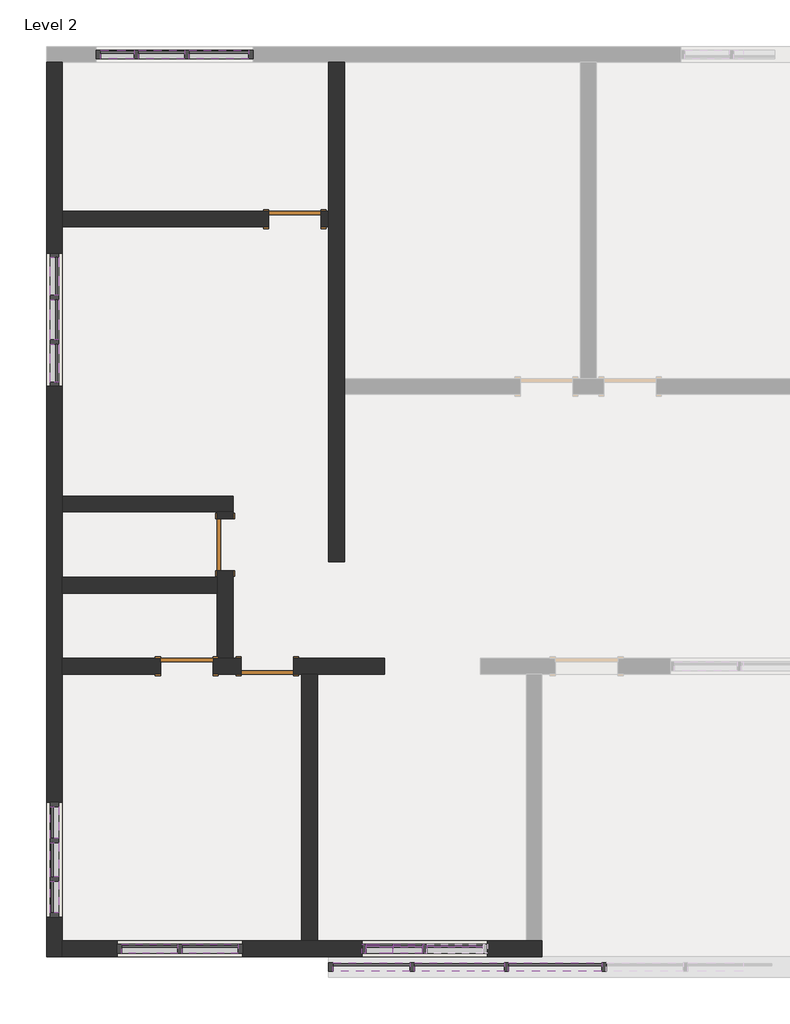
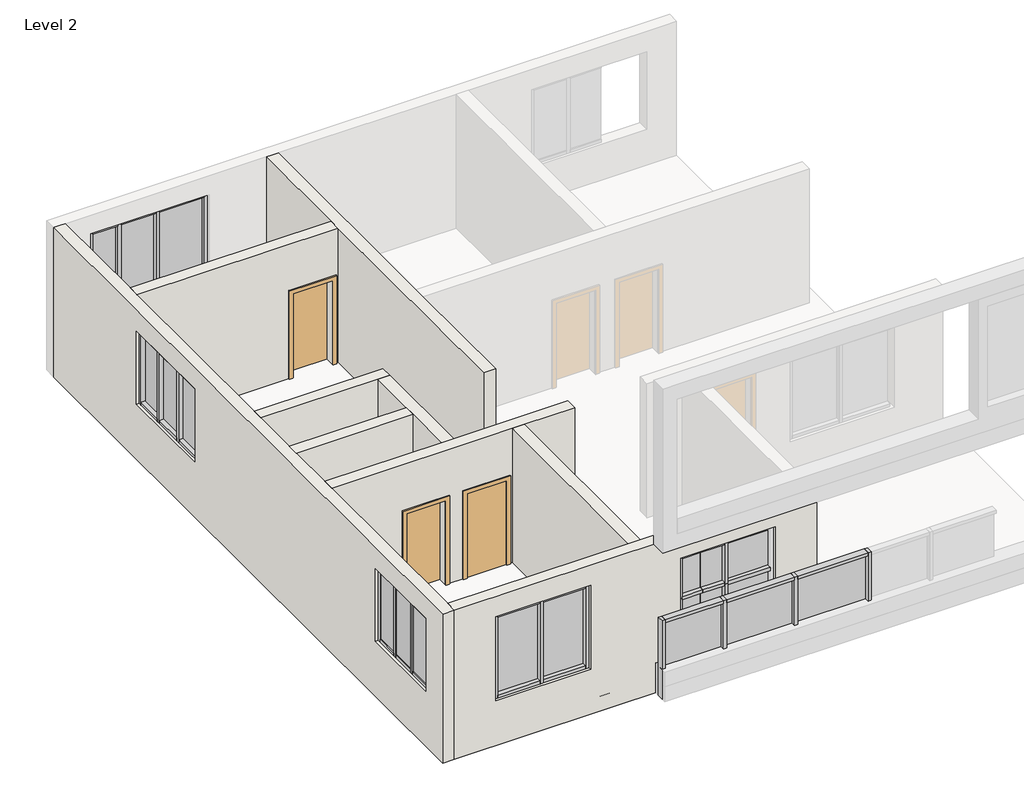
# One storey, part 1 of 2: 56 members, 20 plates, 9 walls, 4 doors.
"""IFC4 building model written with IfcOpenShell, lengths in millimetres."""

from ifc_helpers import new_model, si_unit, frame, origin, place, context, project, spatial, polyline, outline, extrude, faceted_brep, transform, mapped, element, save
from components import door_a1484949, door_85036156, member_c17f1be2, member_ad567e07, member_5535eeb3, member_2ebf4a73, member_b9f3750b, member_051277f3, member_024c663a, member_e254c550, member_3fd136ac, member_73c075c8, member_623bfa76, member_6049e8cb, member_177cc448, member_bc64557a, member_c85333fa, member_70b87a21, member_5e57c25a, member_84b97a81, member_951753a7, member_7096a90e, member_0adfe7f4, member_3d200c31, member_5d841d64, member_75b26f99, member_e6b9f524, member_001188f2, member_d37749d9, member_0d0414c4, system_panel_glazed_b96e00cd, system_panel_glazed_b203cd48, system_panel_glazed_f5076819, system_panel_glazed_6dadbfa4, system_panel_glazed_18fdb1ad, system_panel_glazed_5b9b0e9e, system_panel_glazed_bdb83165, system_panel_glazed_79b80f84, system_panel_glazed_c1c9c451, system_panel_glazed_831e08d1, system_panel_glazed_30877d7e, system_panel_glazed_de05bfa4, system_panel_glazed_4af92da9, system_panel_glazed_616dcef8

model = new_model("IFC4")

# Units and contexts
model_context = context("Model", 3, world=origin())
ifc_project = project(units=[si_unit("LENGTHUNIT", "METRE", prefix="MILLI")], contexts=[model_context])

# Site, building, storey
site = spatial("IfcSite", under=ifc_project)
building = spatial("IfcBuilding", under=site)
storey = spatial("IfcBuildingStorey", under=building, Name="Level 2", Elevation=3048.0)

# Doors
placement = place(None, origin())
door_shape = door_a1484949(model_context)
element("IfcDoor", 1, ObjectType="Single-Flush : 30\" x 80\"", at=placement, inside=storey, context=model_context, shape_type="MappedRepresentation", body=[
    mapped(door_shape, transform((-16666.091855, -3109.9538163, 3048.0), x_axis=(1.0, 0.0, 0.0), y_axis=(0.0, 1.0, 0.0), z_axis=(0.0, 0.0, 1.0))),
])
element("IfcDoor", 2, ObjectType="Single-Flush : 30\" x 80\"", at=placement, inside=storey, context=model_context, shape_type="MappedRepresentation", body=[
    mapped(door_shape, transform((-18240.891855, -9625.0538163, 3048.0), x_axis=(1.0, 0.0, 0.0), y_axis=(0.0, 1.0, 0.0), z_axis=(0.0, 0.0, 1.0))),
])
door_2_shape = door_85036156(model_context)
element("IfcDoor", 3, ObjectType="Single-Flush : 30\" x 80\"", at=placement, inside=storey, context=model_context, shape_type="MappedRepresentation", body=[
    mapped(door_2_shape, transform((-17682.091855, -7853.4038163, 3048.0), x_axis=(0.0, -1.0, 0.0), y_axis=(1.0, 0.0, 0.0), z_axis=(0.0, 0.0, 1.0))),
])
element("IfcDoor", 4, ObjectType="Single-Flush : 30\" x 80\"", at=placement, inside=storey, context=model_context, shape_type="MappedRepresentation", body=[
    mapped(door_2_shape, transform((-17066.141855, -9625.0538163, 3048.0), x_axis=(1.0, 0.0, 0.0), y_axis=(0.0, 1.0, 0.0), z_axis=(0.0, 0.0, 1.0))),
])

# Members
member_shape = member_c17f1be2(model_context)
element("IfcMember", 5, ObjectType="Rectangular Mullion : 2.5\" x 5\" rectangular", at=placement, inside=storey, context=model_context, shape_type="MappedRepresentation", body=[
    mapped(member_shape, transform((-18374.241855, -13739.8538163, 5684.1406455), x_axis=(0.0, 0.0, 1.0), y_axis=(0.0, -1.0, 0.0), z_axis=(1.0, 0.0, 0.0))),
])
element("IfcMember", 6, ObjectType="Rectangular Mullion : 2.5\" x 5\" rectangular", at=placement, inside=storey, context=model_context, shape_type="MappedRepresentation", body=[
    mapped(member_shape, transform((-17491.591855, -13739.8538163, 5684.1406455), x_axis=(0.0, 0.0, 1.0), y_axis=(0.0, -1.0, 0.0), z_axis=(1.0, 0.0, 0.0))),
])
member_2_shape = member_ad567e07(model_context)
element("IfcMember", 7, ObjectType="Rectangular Mullion : 2.5\" x 5\" rectangular", at=placement, inside=storey, context=model_context, shape_type="MappedRepresentation", body=[
    mapped(member_2_shape, transform((-13922.891855, -13739.8538163, 4760.0253323), x_axis=(0.0, 0.0, 1.0), y_axis=(0.0, -1.0, 0.0), z_axis=(1.0, 0.0, 0.0))),
])
element("IfcMember", 8, ObjectType="Rectangular Mullion : 2.5\" x 5\" rectangular", at=placement, inside=storey, context=model_context, shape_type="MappedRepresentation", body=[
    mapped(member_shape, transform((-14742.041855, -13739.8538163, 3888.7401376), x_axis=(0.0, 0.0, -1.0), y_axis=(0.0, -1.0, 0.0), z_axis=(-1.0, 0.0, 0.0))),
])
element("IfcMember", 9, ObjectType="Rectangular Mullion : 2.5\" x 5\" rectangular", at=placement, inside=storey, context=model_context, shape_type="MappedRepresentation", body=[
    mapped(member_shape, transform((-18310.741855, -13739.8538163, 3967.0387154), x_axis=(0.0, 0.0, -1.0), y_axis=(0.0, -1.0, 0.0), z_axis=(-1.0, 0.0, 0.0))),
])
element("IfcMember", 10, ObjectType="Rectangular Mullion : 2.5\" x 5\" rectangular", at=placement, inside=storey, context=model_context, shape_type="MappedRepresentation", body=[
    mapped(member_shape, transform((-19193.391855, -13739.8538163, 3967.0387154), x_axis=(0.0, 0.0, -1.0), y_axis=(0.0, -1.0, 0.0), z_axis=(-1.0, 0.0, 0.0))),
])
member_3_shape = member_5535eeb3(model_context)
element("IfcMember", 11, ObjectType="Rectangular Mullion : 2.5\" x 5\" rectangular", at=placement, inside=storey, context=model_context, shape_type="MappedRepresentation", body=[
    mapped(member_3_shape, transform((-20171.291855, -12755.6038163, 5664.075508), x_axis=(0.0, 0.0, 1.0), y_axis=(1.0, 0.0, 0.0), z_axis=(0.0, 1.0, 0.0))),
])
element("IfcMember", 12, ObjectType="Rectangular Mullion : 2.5\" x 5\" rectangular", at=placement, inside=storey, context=model_context, shape_type="MappedRepresentation", body=[
    mapped(member_3_shape, transform((-20171.291855, -11669.7538163, 5664.075508), x_axis=(0.0, 0.0, 1.0), y_axis=(1.0, 0.0, 0.0), z_axis=(0.0, 1.0, 0.0))),
])
member_4_shape = member_2ebf4a73(model_context)
element("IfcMember", 13, ObjectType="Rectangular Mullion : 2.5\" x 5\" rectangular", at=placement, inside=storey, context=model_context, shape_type="MappedRepresentation", body=[
    mapped(member_4_shape, transform((-20171.291855, -12196.8038163, 5664.075508), x_axis=(0.0, 0.0, 1.0), y_axis=(1.0, 0.0, 0.0), z_axis=(0.0, 1.0, 0.0))),
])
element("IfcMember", 14, ObjectType="Rectangular Mullion : 2.5\" x 5\" rectangular", at=placement, inside=storey, context=model_context, shape_type="MappedRepresentation", body=[
    mapped(member_4_shape, transform((-20171.291855, -12692.1038163, 4177.2250348), x_axis=(0.0, 0.0, -1.0), y_axis=(1.0, 0.0, 0.0), z_axis=(0.0, -1.0, 0.0))),
])
element("IfcMember", 15, ObjectType="Rectangular Mullion : 2.5\" x 5\" rectangular", at=placement, inside=storey, context=model_context, shape_type="MappedRepresentation", body=[
    mapped(member_3_shape, transform((-20171.291855, -12133.3038163, 4177.2250348), x_axis=(0.0, 0.0, -1.0), y_axis=(1.0, 0.0, 0.0), z_axis=(0.0, -1.0, 0.0))),
])
element("IfcMember", 16, ObjectType="Rectangular Mullion : 2.5\" x 5\" rectangular", at=placement, inside=storey, context=model_context, shape_type="MappedRepresentation", body=[
    mapped(member_3_shape, transform((-20171.291855, -13219.1538163, 4177.2250348), x_axis=(0.0, 0.0, -1.0), y_axis=(1.0, 0.0, 0.0), z_axis=(0.0, -1.0, 0.0))),
])
member_5_shape = member_b9f3750b(model_context)
element("IfcMember", 17, ObjectType="Rectangular Mullion : 2.5\" x 5\" rectangular", at=placement, inside=storey, context=model_context, shape_type="MappedRepresentation", body=[
    mapped(member_5_shape, transform((-19009.241855, -709.6538163, 5710.0962507), x_axis=(0.0, 0.0, 1.0), y_axis=(0.0, -1.0, 0.0), z_axis=(1.0, 0.0, 0.0))),
])
member_6_shape = member_051277f3(model_context)
element("IfcMember", 18, ObjectType="Rectangular Mullion : 2.5\" x 5\" rectangular", at=placement, inside=storey, context=model_context, shape_type="MappedRepresentation", body=[
    mapped(member_6_shape, transform((-18272.641855, -709.6538163, 5710.0962507), x_axis=(0.0, 0.0, 1.0), y_axis=(0.0, -1.0, 0.0), z_axis=(1.0, 0.0, 0.0))),
])
member_7_shape = member_024c663a(model_context)
element("IfcMember", 19, ObjectType="Rectangular Mullion : 2.5\" x 5\" rectangular", at=placement, inside=storey, context=model_context, shape_type="MappedRepresentation", body=[
    mapped(member_7_shape, transform((-17339.191855, -709.6538163, 5710.0962507), x_axis=(0.0, 0.0, 1.0), y_axis=(0.0, -1.0, 0.0), z_axis=(1.0, 0.0, 0.0))),
])
member_8_shape = member_e254c550(model_context)
element("IfcMember", 20, ObjectType="Rectangular Mullion : 2.5\" x 5\" rectangular", at=placement, inside=storey, context=model_context, shape_type="MappedRepresentation", body=[
    mapped(member_8_shape, transform((-18240.891855, -709.6538163, 4156.5855814), x_axis=(1.0, 0.0, 0.0), y_axis=(0.0, -1.0, 0.0), z_axis=(0.0, 0.0, -1.0))),
])
element("IfcMember", 21, ObjectType="Rectangular Mullion : 2.5\" x 5\" rectangular", at=placement, inside=storey, context=model_context, shape_type="MappedRepresentation", body=[
    mapped(member_8_shape, transform((-18977.491855, -709.6538163, 4156.5855814), x_axis=(1.0, 0.0, 0.0), y_axis=(0.0, -1.0, 0.0), z_axis=(0.0, 0.0, -1.0))),
])
element("IfcMember", 22, ObjectType="Rectangular Mullion : 2.5\" x 5\" rectangular", at=placement, inside=storey, context=model_context, shape_type="MappedRepresentation", body=[
    mapped(member_6_shape, transform((-18945.741855, -709.6538163, 4156.5855814), x_axis=(0.0, 0.0, -1.0), y_axis=(0.0, -1.0, 0.0), z_axis=(-1.0, 0.0, 0.0))),
])
element("IfcMember", 23, ObjectType="Rectangular Mullion : 2.5\" x 5\" rectangular", at=placement, inside=storey, context=model_context, shape_type="MappedRepresentation", body=[
    mapped(member_7_shape, transform((-18209.141855, -709.6538163, 4156.5855814), x_axis=(0.0, 0.0, -1.0), y_axis=(0.0, -1.0, 0.0), z_axis=(-1.0, 0.0, 0.0))),
])
element("IfcMember", 24, ObjectType="Rectangular Mullion : 2.5\" x 5\" rectangular", at=placement, inside=storey, context=model_context, shape_type="MappedRepresentation", body=[
    mapped(member_5_shape, transform((-19498.191855, -709.6538163, 4156.5855814), x_axis=(0.0, 0.0, -1.0), y_axis=(0.0, -1.0, 0.0), z_axis=(-1.0, 0.0, 0.0))),
])
member_9_shape = member_3fd136ac(model_context)
element("IfcMember", 25, ObjectType="Rectangular Mullion : 2.5\" x 5\" rectangular", at=placement, inside=storey, context=model_context, shape_type="MappedRepresentation", body=[
    mapped(member_9_shape, transform((-19561.691855, -709.6538163, 5710.0962507), x_axis=(-1.0, 0.0, 0.0), y_axis=(0.0, -1.0, 0.0), z_axis=(0.0, 0.0, 1.0))),
])
element("IfcMember", 26, ObjectType="Rectangular Mullion : 2.5\" x 5\" rectangular", at=placement, inside=storey, context=model_context, shape_type="MappedRepresentation", body=[
    mapped(member_9_shape, transform((-17275.691855, -709.6538163, 4156.5855814), x_axis=(1.0, 0.0, 0.0), y_axis=(0.0, -1.0, 0.0), z_axis=(0.0, 0.0, -1.0))),
])
member_10_shape = member_73c075c8(model_context)
element("IfcMember", 27, ObjectType="Rectangular Mullion : 2.5\" x 5\" rectangular", at=placement, inside=storey, context=model_context, shape_type="MappedRepresentation", body=[
    mapped(member_10_shape, transform((-20171.291855, -4932.4038163, 4168.0644408), x_axis=(0.0, 0.0, -1.0), y_axis=(-1.0, 0.0, 0.0), z_axis=(0.0, 1.0, 0.0))),
])
element("IfcMember", 28, ObjectType="Rectangular Mullion : 2.5\" x 5\" rectangular", at=placement, inside=storey, context=model_context, shape_type="MappedRepresentation", body=[
    mapped(member_10_shape, transform((-20171.291855, -3668.7538163, 4168.0644408), x_axis=(0.0, 0.0, -1.0), y_axis=(-1.0, 0.0, 0.0), z_axis=(0.0, 1.0, 0.0))),
])
member_11_shape = member_623bfa76(model_context)
element("IfcMember", 29, ObjectType="Rectangular Mullion : 2.5\" x 5\" rectangular", at=placement, inside=storey, context=model_context, shape_type="MappedRepresentation", body=[
    mapped(member_11_shape, transform((-20171.291855, -4284.7038163, 4168.0644408), x_axis=(0.0, 0.0, -1.0), y_axis=(-1.0, 0.0, 0.0), z_axis=(0.0, 1.0, 0.0))),
])
member_12_shape = member_6049e8cb(model_context)
element("IfcMember", 30, ObjectType="Rectangular Mullion : 2.5\" x 5\" rectangular", at=placement, inside=storey, context=model_context, shape_type="MappedRepresentation", body=[
    mapped(member_12_shape, transform((-20171.291855, -4900.6538163, 4168.0644408), x_axis=(0.0, -1.0, 0.0), y_axis=(-1.0, 0.0, 0.0), z_axis=(0.0, 0.0, -1.0))),
])
element("IfcMember", 31, ObjectType="Rectangular Mullion : 2.5\" x 5\" rectangular", at=placement, inside=storey, context=model_context, shape_type="MappedRepresentation", body=[
    mapped(member_12_shape, transform((-20171.291855, -4252.9538163, 4168.0644408), x_axis=(0.0, -1.0, 0.0), y_axis=(-1.0, 0.0, 0.0), z_axis=(0.0, 0.0, -1.0))),
])
element("IfcMember", 32, ObjectType="Rectangular Mullion : 2.5\" x 5\" rectangular", at=placement, inside=storey, context=model_context, shape_type="MappedRepresentation", body=[
    mapped(member_11_shape, transform((-20171.291855, -4868.9038163, 5661.6118891), x_axis=(0.0, 0.0, 1.0), y_axis=(-1.0, 0.0, 0.0), z_axis=(0.0, -1.0, 0.0))),
])
element("IfcMember", 33, ObjectType="Rectangular Mullion : 2.5\" x 5\" rectangular", at=placement, inside=storey, context=model_context, shape_type="MappedRepresentation", body=[
    mapped(member_10_shape, transform((-20171.291855, -4221.2038163, 5661.6118891), x_axis=(0.0, 0.0, 1.0), y_axis=(-1.0, 0.0, 0.0), z_axis=(0.0, -1.0, 0.0))),
])
element("IfcMember", 34, ObjectType="Rectangular Mullion : 2.5\" x 5\" rectangular", at=placement, inside=storey, context=model_context, shape_type="MappedRepresentation", body=[
    mapped(member_10_shape, transform((-20171.291855, -5484.8538163, 5661.6118891), x_axis=(0.0, 0.0, 1.0), y_axis=(-1.0, 0.0, 0.0), z_axis=(0.0, -1.0, 0.0))),
])
member_13_shape = member_177cc448(model_context)
element("IfcMember", 35, ObjectType="Rectangular Mullion : 2.5\" x 5\" rectangular", at=placement, inside=storey, context=model_context, shape_type="MappedRepresentation", body=[
    mapped(member_13_shape, transform((-20171.291855, -5548.3538163, 4168.0644408), x_axis=(0.0, -1.0, 0.0), y_axis=(-1.0, 0.0, 0.0), z_axis=(0.0, 0.0, -1.0))),
])
element("IfcMember", 36, ObjectType="Rectangular Mullion : 2.5\" x 5\" rectangular", at=placement, inside=storey, context=model_context, shape_type="MappedRepresentation", body=[
    mapped(member_13_shape, transform((-20171.291855, -3605.2538163, 5661.6118891), x_axis=(0.0, 1.0, 0.0), y_axis=(-1.0, 0.0, 0.0), z_axis=(0.0, 0.0, 1.0))),
])
member_14_shape = member_bc64557a(model_context)
element("IfcMember", 37, ObjectType="Rectangular Mullion : 2.5\" x 5\" rectangular", at=placement, inside=storey, context=model_context, shape_type="MappedRepresentation", body=[
    mapped(member_14_shape, transform((-20171.291855, -12165.0538163, 4177.2250348), x_axis=(0.0, 1.0, 0.0), y_axis=(1.0, 0.0, 0.0), z_axis=(0.0, 0.0, -1.0))),
])
element("IfcMember", 38, ObjectType="Rectangular Mullion : 2.5\" x 5\" rectangular", at=placement, inside=storey, context=model_context, shape_type="MappedRepresentation", body=[
    mapped(member_14_shape, transform((-20171.291855, -12723.8538163, 4177.2250348), x_axis=(0.0, 1.0, 0.0), y_axis=(1.0, 0.0, 0.0), z_axis=(0.0, 0.0, -1.0))),
])
member_15_shape = member_c85333fa(model_context)
element("IfcMember", 39, ObjectType="Rectangular Mullion : 2.5\" x 5\" rectangular", at=placement, inside=storey, context=model_context, shape_type="MappedRepresentation", body=[
    mapped(member_15_shape, transform((-20171.291855, -13282.6538163, 5664.075508), x_axis=(0.0, -1.0, 0.0), y_axis=(1.0, 0.0, 0.0), z_axis=(0.0, 0.0, 1.0))),
])
element("IfcMember", 40, ObjectType="Rectangular Mullion : 2.5\" x 5\" rectangular", at=placement, inside=storey, context=model_context, shape_type="MappedRepresentation", body=[
    mapped(member_15_shape, transform((-20171.291855, -11606.2538163, 4177.2250348), x_axis=(0.0, 1.0, 0.0), y_axis=(1.0, 0.0, 0.0), z_axis=(0.0, 0.0, -1.0))),
])
member_16_shape = member_70b87a21(model_context)
element("IfcMember", 41, ObjectType="Rectangular Mullion : 2.5\" x 5\" rectangular", at=placement, inside=storey, context=model_context, shape_type="MappedRepresentation", body=[
    mapped(member_16_shape, transform((-14805.541855, -13739.8538163, 4760.0253323), x_axis=(0.0, 0.0, 1.0), y_axis=(0.0, -1.0, 0.0), z_axis=(1.0, 0.0, 0.0))),
])
member_17_shape = member_5e57c25a(model_context)
element("IfcMember", 42, ObjectType="Rectangular Mullion : 2.5\" x 5\" rectangular", at=placement, inside=storey, context=model_context, shape_type="MappedRepresentation", body=[
    mapped(member_17_shape, transform((-14773.791855, -13739.8538163, 4760.0253323), x_axis=(1.0, 0.0, 0.0), y_axis=(0.0, -1.0, 0.0), z_axis=(0.0, 0.0, -1.0))),
])
member_18_shape = member_84b97a81(model_context)
element("IfcMember", 43, ObjectType="Rectangular Mullion : 2.5\" x 5\" rectangular", at=placement, inside=storey, context=model_context, shape_type="MappedRepresentation", body=[
    mapped(member_18_shape, transform((-14805.541855, -13739.8538163, 5631.310527), x_axis=(0.0, 0.0, 1.0), y_axis=(0.0, -1.0, 0.0), z_axis=(1.0, 0.0, 0.0))),
])
element("IfcMember", 44, ObjectType="Rectangular Mullion : 2.5\" x 5\" rectangular", at=placement, inside=storey, context=model_context, shape_type="MappedRepresentation", body=[
    mapped(member_17_shape, transform((-14773.791855, -13739.8538163, 3888.7401376), x_axis=(1.0, 0.0, 0.0), y_axis=(0.0, -1.0, 0.0), z_axis=(0.0, 0.0, -1.0))),
])
element("IfcMember", 45, ObjectType="Rectangular Mullion : 2.5\" x 5\" rectangular", at=placement, inside=storey, context=model_context, shape_type="MappedRepresentation", body=[
    mapped(member_18_shape, transform((-15230.991855, -13739.8538163, 3888.7401376), x_axis=(0.0, 0.0, -1.0), y_axis=(0.0, -1.0, 0.0), z_axis=(-1.0, 0.0, 0.0))),
])
member_19_shape = member_951753a7(model_context)
element("IfcMember", 46, ObjectType="Rectangular Mullion : 2.5\" x 5\" rectangular", at=placement, inside=storey, context=model_context, shape_type="MappedRepresentation", body=[
    mapped(member_19_shape, transform((-15230.991855, -13739.8538163, 4760.0253323), x_axis=(0.0, 0.0, 1.0), y_axis=(0.0, -1.0, 0.0), z_axis=(1.0, 0.0, 0.0))),
])
member_20_shape = member_7096a90e(model_context)
element("IfcMember", 47, ObjectType="Rectangular Mullion : 2.5\" x 5\" rectangular", at=placement, inside=storey, context=model_context, shape_type="MappedRepresentation", body=[
    mapped(member_20_shape, transform((-15230.991855, -13739.8538163, 5631.310527), x_axis=(0.0, 0.0, 1.0), y_axis=(0.0, -1.0, 0.0), z_axis=(1.0, 0.0, 0.0))),
])
element("IfcMember", 48, ObjectType="Rectangular Mullion : 2.5\" x 5\" rectangular", at=placement, inside=storey, context=model_context, shape_type="MappedRepresentation", body=[
    mapped(member_20_shape, transform((-15624.691855, -13739.8538163, 3888.7401376), x_axis=(0.0, 0.0, -1.0), y_axis=(0.0, -1.0, 0.0), z_axis=(-1.0, 0.0, 0.0))),
])
member_21_shape = member_0adfe7f4(model_context)
element("IfcMember", 49, ObjectType="Rectangular Mullion : 2.5\" x 5\" rectangular", at=placement, inside=storey, context=model_context, shape_type="MappedRepresentation", body=[
    mapped(member_21_shape, transform((-15688.191855, -13739.8538163, 4760.0253323), x_axis=(-1.0, 0.0, 0.0), y_axis=(0.0, -1.0, 0.0), z_axis=(0.0, 0.0, 1.0))),
])
element("IfcMember", 50, ObjectType="Rectangular Mullion : 2.5\" x 5\" rectangular", at=placement, inside=storey, context=model_context, shape_type="MappedRepresentation", body=[
    mapped(member_21_shape, transform((-15688.191855, -13739.8538163, 5631.310527), x_axis=(-1.0, 0.0, 0.0), y_axis=(0.0, -1.0, 0.0), z_axis=(0.0, 0.0, 1.0))),
])
member_22_shape = member_3d200c31(model_context)
element("IfcMember", 51, ObjectType="Rectangular Mullion : 2.5\" x 5\" rectangular", at=placement, inside=storey, context=model_context, shape_type="MappedRepresentation", body=[
    mapped(member_22_shape, transform((-18342.491855, -13739.8538163, 3967.0387154), x_axis=(1.0, 0.0, 0.0), y_axis=(0.0, -1.0, 0.0), z_axis=(0.0, 0.0, -1.0))),
])
member_23_shape = member_5d841d64(model_context)
element("IfcMember", 52, ObjectType="Rectangular Mullion : 2.5\" x 5\" rectangular", at=placement, inside=storey, context=model_context, shape_type="MappedRepresentation", body=[
    mapped(member_23_shape, transform((-17428.091855, -13739.8538163, 3967.0387154), x_axis=(1.0, 0.0, 0.0), y_axis=(0.0, -1.0, 0.0), z_axis=(0.0, 0.0, -1.0))),
])
element("IfcMember", 53, ObjectType="Rectangular Mullion : 2.5\" x 5\" rectangular", at=placement, inside=storey, context=model_context, shape_type="MappedRepresentation", body=[
    mapped(member_23_shape, transform((-19256.891855, -13739.8538163, 5684.1406455), x_axis=(-1.0, 0.0, 0.0), y_axis=(0.0, -1.0, 0.0), z_axis=(0.0, 0.0, 1.0))),
])
member_24_shape = member_75b26f99(model_context)
element("IfcMember", 54, ObjectType="Rectangular Mullion : 2.5\" x 5\" rectangular", at=placement, inside=storey, context=model_context, shape_type="MappedRepresentation", body=[
    mapped(member_24_shape, transform((-16170.791855, -14006.5538163, 4647.2829369), x_axis=(-1.0, 0.0, 0.0), y_axis=(0.0, -1.0, 0.0), z_axis=(0.0, 0.0, 1.0))),
])
member_25_shape = member_e6b9f524(model_context)
element("IfcMember", 55, ObjectType="Rectangular Mullion : 2.5\" x 5\" rectangular", at=placement, inside=storey, context=model_context, shape_type="MappedRepresentation", body=[
    mapped(member_25_shape, transform((-14983.341855, -14006.5538163, 4647.2829369), x_axis=(0.0, 0.0, 1.0), y_axis=(0.0, -1.0, 0.0), z_axis=(1.0, 0.0, 0.0))),
])
member_26_shape = member_001188f2(model_context)
element("IfcMember", 56, ObjectType="Rectangular Mullion : 2.5\" x 5\" rectangular", at=placement, inside=storey, context=model_context, shape_type="MappedRepresentation", body=[
    mapped(member_26_shape, transform((-14951.591855, -14006.5538163, 3048.0), x_axis=(1.0, 0.0, 0.0), y_axis=(0.0, -1.0, 0.0), z_axis=(0.0, 0.0, -1.0))),
])
element("IfcMember", 57, ObjectType="Rectangular Mullion : 2.5\" x 5\" rectangular", at=placement, inside=storey, context=model_context, shape_type="MappedRepresentation", body=[
    mapped(member_26_shape, transform((-13579.991855, -14006.5538163, 3048.0), x_axis=(1.0, 0.0, 0.0), y_axis=(0.0, -1.0, 0.0), z_axis=(0.0, 0.0, -1.0))),
])
element("IfcMember", 58, ObjectType="Rectangular Mullion : 2.5\" x 5\" rectangular", at=placement, inside=storey, context=model_context, shape_type="MappedRepresentation", body=[
    mapped(member_26_shape, transform((-12157.591855, -14006.5538163, 3048.0), x_axis=(1.0, 0.0, 0.0), y_axis=(0.0, -1.0, 0.0), z_axis=(0.0, 0.0, -1.0))),
])
member_27_shape = member_d37749d9(model_context)
element("IfcMember", 59, ObjectType="Rectangular Mullion : 2.5\" x 5\" rectangular", at=placement, inside=storey, context=model_context, shape_type="MappedRepresentation", body=[
    mapped(member_27_shape, transform((-13611.741855, -14006.5538163, 4647.2829369), x_axis=(0.0, 0.0, 1.0), y_axis=(0.0, -1.0, 0.0), z_axis=(1.0, 0.0, 0.0))),
])
member_28_shape = member_0d0414c4(model_context)
element("IfcMember", 60, ObjectType="Rectangular Mullion : 2.5\" x 5\" rectangular", at=placement, inside=storey, context=model_context, shape_type="MappedRepresentation", body=[
    mapped(member_28_shape, transform((-12189.341855, -14006.5538163, 4647.2829369), x_axis=(0.0, 0.0, 1.0), y_axis=(0.0, -1.0, 0.0), z_axis=(1.0, 0.0, 0.0))),
])

# Plates
system_panel_glazed_shape = system_panel_glazed_b96e00cd(model_context)
element("IfcPlate", 61, ObjectType="System Panel : Glazed", at=placement, inside=storey, context=model_context, shape_type="MappedRepresentation", body=[
    mapped(system_panel_glazed_shape, transform((-19253.716855, -709.6538163, 4220.0855814), x_axis=(1.0, 0.0, 0.0), y_axis=(0.0, 1.0, 0.0), z_axis=(0.0, 0.0, 1.0))),
])
system_panel_glazed_2_shape = system_panel_glazed_b203cd48(model_context)
element("IfcPlate", 62, ObjectType="System Panel : Glazed", at=placement, inside=storey, context=model_context, shape_type="MappedRepresentation", body=[
    mapped(system_panel_glazed_2_shape, transform((-17774.166855, -709.6538163, 4220.0855814), x_axis=(1.0, 0.0, 0.0), y_axis=(0.0, 1.0, 0.0), z_axis=(0.0, 0.0, 1.0))),
])
system_panel_glazed_3_shape = system_panel_glazed_f5076819(model_context)
element("IfcPlate", 63, ObjectType="System Panel : Glazed", at=placement, inside=storey, context=model_context, shape_type="MappedRepresentation", body=[
    mapped(system_panel_glazed_3_shape, transform((-18609.191855, -709.6538163, 4220.0855814), x_axis=(1.0, 0.0, 0.0), y_axis=(0.0, 1.0, 0.0), z_axis=(0.0, 0.0, 1.0))),
])
system_panel_glazed_4_shape = system_panel_glazed_6dadbfa4(model_context)
element("IfcPlate", 64, ObjectType="System Panel : Glazed", at=placement, inside=storey, context=model_context, shape_type="MappedRepresentation", body=[
    mapped(system_panel_glazed_4_shape, transform((-20171.291855, -3944.9788163, 4231.5644408), x_axis=(0.0, -1.0, 0.0), y_axis=(1.0, 0.0, 0.0), z_axis=(0.0, 0.0, 1.0))),
])
element("IfcPlate", 65, ObjectType="System Panel : Glazed", at=placement, inside=storey, context=model_context, shape_type="MappedRepresentation", body=[
    mapped(system_panel_glazed_4_shape, transform((-20171.291855, -5208.6288163, 4231.5644408), x_axis=(0.0, -1.0, 0.0), y_axis=(1.0, 0.0, 0.0), z_axis=(0.0, 0.0, 1.0))),
])
system_panel_glazed_5_shape = system_panel_glazed_18fdb1ad(model_context)
element("IfcPlate", 66, ObjectType="System Panel : Glazed", at=placement, inside=storey, context=model_context, shape_type="MappedRepresentation", body=[
    mapped(system_panel_glazed_5_shape, transform((-20171.291855, -4576.8038163, 4231.5644408), x_axis=(0.0, -1.0, 0.0), y_axis=(1.0, 0.0, 0.0), z_axis=(0.0, 0.0, 1.0))),
])
system_panel_glazed_6_shape = system_panel_glazed_5b9b0e9e(model_context)
element("IfcPlate", 67, ObjectType="System Panel : Glazed", at=placement, inside=storey, context=model_context, shape_type="MappedRepresentation", body=[
    mapped(system_panel_glazed_6_shape, transform((-20171.291855, -12987.3788163, 4240.7250348), x_axis=(0.0, 1.0, 0.0), y_axis=(-1.0, 0.0, 0.0), z_axis=(0.0, 0.0, 1.0))),
])
element("IfcPlate", 68, ObjectType="System Panel : Glazed", at=placement, inside=storey, context=model_context, shape_type="MappedRepresentation", body=[
    mapped(system_panel_glazed_6_shape, transform((-20171.291855, -11901.5288163, 4240.7250348), x_axis=(0.0, 1.0, 0.0), y_axis=(-1.0, 0.0, 0.0), z_axis=(0.0, 0.0, 1.0))),
])
system_panel_glazed_7_shape = system_panel_glazed_bdb83165(model_context)
element("IfcPlate", 69, ObjectType="System Panel : Glazed", at=placement, inside=storey, context=model_context, shape_type="MappedRepresentation", body=[
    mapped(system_panel_glazed_7_shape, transform((-20171.291855, -12444.4538163, 4240.7250348), x_axis=(0.0, 1.0, 0.0), y_axis=(-1.0, 0.0, 0.0), z_axis=(0.0, 0.0, 1.0))),
])
system_panel_glazed_8_shape = system_panel_glazed_79b80f84(model_context)
element("IfcPlate", 70, ObjectType="System Panel : Glazed", at=placement, inside=storey, context=model_context, shape_type="MappedRepresentation", body=[
    mapped(system_panel_glazed_8_shape, transform((-15018.266855, -13739.8538163, 3952.2401376), x_axis=(1.0, 0.0, 0.0), y_axis=(0.0, 1.0, 0.0), z_axis=(0.0, 0.0, 1.0))),
])
element("IfcPlate", 71, ObjectType="System Panel : Glazed", at=placement, inside=storey, context=model_context, shape_type="MappedRepresentation", body=[
    mapped(system_panel_glazed_8_shape, transform((-15018.266855, -13739.8538163, 4791.7753323), x_axis=(1.0, 0.0, 0.0), y_axis=(0.0, 1.0, 0.0), z_axis=(0.0, 0.0, 1.0))),
])
system_panel_glazed_9_shape = system_panel_glazed_c1c9c451(model_context)
element("IfcPlate", 72, ObjectType="System Panel : Glazed", at=placement, inside=storey, context=model_context, shape_type="MappedRepresentation", body=[
    mapped(system_panel_glazed_9_shape, transform((-14332.466855, -13739.8538163, 3952.2401376), x_axis=(1.0, 0.0, 0.0), y_axis=(0.0, 1.0, 0.0), z_axis=(0.0, 0.0, 1.0))),
])
element("IfcPlate", 73, ObjectType="System Panel : Glazed", at=placement, inside=storey, context=model_context, shape_type="MappedRepresentation", body=[
    mapped(system_panel_glazed_9_shape, transform((-14332.466855, -13739.8538163, 4791.7753323), x_axis=(1.0, 0.0, 0.0), y_axis=(0.0, 1.0, 0.0), z_axis=(0.0, 0.0, 1.0))),
])
system_panel_glazed_10_shape = system_panel_glazed_831e08d1(model_context)
element("IfcPlate", 74, ObjectType="System Panel : Glazed", at=placement, inside=storey, context=model_context, shape_type="MappedRepresentation", body=[
    mapped(system_panel_glazed_10_shape, transform((-15427.841855, -13739.8538163, 3952.2401376), x_axis=(1.0, 0.0, 0.0), y_axis=(0.0, 1.0, 0.0), z_axis=(0.0, 0.0, 1.0))),
])
element("IfcPlate", 75, ObjectType="System Panel : Glazed", at=placement, inside=storey, context=model_context, shape_type="MappedRepresentation", body=[
    mapped(system_panel_glazed_10_shape, transform((-15427.841855, -13739.8538163, 4791.7753323), x_axis=(1.0, 0.0, 0.0), y_axis=(0.0, 1.0, 0.0), z_axis=(0.0, 0.0, 1.0))),
])
system_panel_glazed_11_shape = system_panel_glazed_30877d7e(model_context)
element("IfcPlate", 76, ObjectType="System Panel : Glazed", at=placement, inside=storey, context=model_context, shape_type="MappedRepresentation", body=[
    mapped(system_panel_glazed_11_shape, transform((-18783.816855, -13739.8538163, 4030.5387154), x_axis=(1.0, 0.0, 0.0), y_axis=(0.0, 1.0, 0.0), z_axis=(0.0, 0.0, 1.0))),
])
element("IfcPlate", 77, ObjectType="System Panel : Glazed", at=placement, inside=storey, context=model_context, shape_type="MappedRepresentation", body=[
    mapped(system_panel_glazed_11_shape, transform((-17901.166855, -13739.8538163, 4030.5387154), x_axis=(1.0, 0.0, 0.0), y_axis=(0.0, 1.0, 0.0), z_axis=(0.0, 0.0, 1.0))),
])
system_panel_glazed_12_shape = system_panel_glazed_de05bfa4(model_context)
element("IfcPlate", 78, ObjectType="System Panel : Glazed", at=placement, inside=storey, context=model_context, shape_type="MappedRepresentation", body=[
    mapped(system_panel_glazed_12_shape, transform((-15545.316855, -14006.5538163, 3048.0), x_axis=(1.0, 0.0, 0.0), y_axis=(0.0, 1.0, 0.0), z_axis=(0.0, 0.0, 1.0))),
])
system_panel_glazed_13_shape = system_panel_glazed_4af92da9(model_context)
element("IfcPlate", 79, ObjectType="System Panel : Glazed", at=placement, inside=storey, context=model_context, shape_type="MappedRepresentation", body=[
    mapped(system_panel_glazed_13_shape, transform((-14265.791855, -14006.5538163, 3048.0), x_axis=(1.0, 0.0, 0.0), y_axis=(0.0, 1.0, 0.0), z_axis=(0.0, 0.0, 1.0))),
])
system_panel_glazed_14_shape = system_panel_glazed_616dcef8(model_context)
element("IfcPlate", 80, ObjectType="System Panel : Glazed", at=placement, inside=storey, context=model_context, shape_type="MappedRepresentation", body=[
    mapped(system_panel_glazed_14_shape, transform((-12868.791855, -14006.5538163, 3048.0), x_axis=(1.0, 0.0, 0.0), y_axis=(0.0, 1.0, 0.0), z_axis=(0.0, 0.0, 1.0))),
])

# Walls
element("IfcWall", 81, ObjectType="9\"", at=placement, inside=storey, context=model_context, shape_type="Brep", body=[
    faceted_brep([(-20285.591855, -823.9538163, 3048.0), (-20285.591855, -13854.1538163, 3048.0), (-20285.591855, -13854.1538163, 6096.0), (-20285.591855, -823.9538163, 6096.0), (-20285.591855, -3605.2538163, 4168.0644408), (-20285.591855, -3605.2538163, 5661.6118891), (-20285.591855, -5548.3538163, 5661.6118891), (-20285.591855, -5548.3538163, 4168.0644408), (-20285.591855, -13282.6538163, 5664.075508), (-20285.591855, -13282.6538163, 4177.2250348), (-20285.591855, -11606.2538163, 4177.2250348), (-20285.591855, -11606.2538163, 5664.075508), (-20056.991855, -13854.1538163, 3048.0), (-20056.991855, -13625.5538163, 3048.0), (-20056.991855, -9739.3538163, 3048.0), (-20056.991855, -9510.7538163, 3048.0), (-20056.991855, -8558.2538163, 3048.0), (-20056.991855, -8329.6538163, 3048.0), (-20056.991855, -7377.1538163, 3048.0), (-20056.991855, -7148.5538163, 3048.0), (-20056.991855, -3224.2538163, 3048.0), (-20056.991855, -2995.6538163, 3048.0), (-20056.991855, -823.9538163, 3048.0), (-20056.991855, -823.9538163, 6096.0), (-20056.991855, -2995.6538163, 6096.0), (-20056.991855, -3224.2538163, 6096.0), (-20056.991855, -7148.5538163, 6096.0), (-20056.991855, -7377.1538163, 6096.0), (-20056.991855, -8329.6538163, 6096.0), (-20056.991855, -8558.2538163, 6096.0), (-20056.991855, -9510.7538163, 6096.0), (-20056.991855, -9739.3538163, 6096.0), (-20056.991855, -13625.5538163, 6096.0), (-20056.991855, -13854.1538163, 6096.0), (-20056.991855, -3605.2538163, 5661.6118891), (-20056.991855, -3605.2538163, 4168.0644408), (-20056.991855, -5548.3538163, 4168.0644408), (-20056.991855, -5548.3538163, 5661.6118891), (-20056.991855, -13282.6538163, 4177.2250348), (-20056.991855, -13282.6538163, 5664.075508), (-20056.991855, -11606.2538163, 5664.075508), (-20056.991855, -11606.2538163, 4177.2250348)], [[[0, 1, 2, 3], [4, 5, 6, 7], [8, 9, 10, 11]], [[12, 13, 14, 15, 16, 17, 18, 19, 20, 21, 22, 23, 24, 25, 26, 27, 28, 29, 30, 31, 32, 33], [34, 35, 36, 37], [38, 39, 40, 41]], [[1, 0, 22, 21, 20, 19, 18, 17, 16, 15, 14, 13, 12]], [[3, 2, 33, 32, 31, 30, 29, 28, 27, 26, 25, 24, 23]], [[0, 3, 23, 22]], [[2, 1, 12, 33]], [[4, 35, 34, 5]], [[5, 34, 37, 6]], [[6, 37, 36, 7]], [[35, 4, 7, 36]], [[38, 9, 8, 39]], [[39, 8, 11, 40]], [[10, 41, 40, 11]], [[9, 38, 41, 10]]]),
])
element("IfcWall", 82, ObjectType="9\"", at=placement, inside=storey, context=model_context, shape_type="Brep", body=[
    faceted_brep([(-13059.291855, -13625.5538163, 3048.0), (-13287.891855, -13625.5538163, 3048.0), (-16335.891855, -13625.5538163, 3048.0), (-16564.491855, -13625.5538163, 3048.0), (-20056.991855, -13625.5538163, 3048.0), (-20056.991855, -13625.5538163, 6096.0), (-16564.491855, -13625.5538163, 6096.0), (-16335.891855, -13625.5538163, 6096.0), (-13287.891855, -13625.5538163, 6096.0), (-13059.291855, -13625.5538163, 6096.0), (-15688.191855, -13625.5538163, 5631.310527), (-15688.191855, -13625.5538163, 3888.7401376), (-13859.391855, -13625.5538163, 3888.7401376), (-13859.391855, -13625.5538163, 5631.310527), (-19256.891855, -13625.5538163, 5684.1406455), (-19256.891855, -13625.5538163, 3967.0387154), (-17428.091855, -13625.5538163, 3967.0387154), (-17428.091855, -13625.5538163, 5684.1406455), (-20056.991855, -13854.1538163, 3048.0), (-13059.291855, -13854.1538163, 3048.0), (-13059.291855, -13854.1538163, 6096.0), (-20056.991855, -13854.1538163, 6096.0), (-15688.191855, -13854.1538163, 3888.7401376), (-15688.191855, -13854.1538163, 5631.310527), (-13859.391855, -13854.1538163, 5631.310527), (-13859.391855, -13854.1538163, 3888.7401376), (-19256.891855, -13854.1538163, 3967.0387154), (-19256.891855, -13854.1538163, 5684.1406455), (-17428.091855, -13854.1538163, 5684.1406455), (-17428.091855, -13854.1538163, 3967.0387154)], [[[0, 1, 2, 3, 4, 5, 6, 7, 8, 9], [10, 11, 12, 13], [14, 15, 16, 17]], [[18, 19, 20, 21], [22, 23, 24, 25], [26, 27, 28, 29]], [[4, 3, 2, 1, 0, 19, 18]], [[9, 8, 7, 6, 5, 21, 20]], [[5, 4, 18, 21]], [[0, 9, 20, 19]], [[10, 23, 22, 11]], [[23, 10, 13, 24]], [[24, 13, 12, 25]], [[11, 22, 25, 12]], [[26, 15, 14, 27]], [[27, 14, 17, 28]], [[28, 17, 16, 29]], [[15, 26, 29, 16]]]),
])
element("IfcWall", 83, ObjectType="9\"", at=placement, inside=storey, context=model_context, shape_type="Brep", body=[
    faceted_brep([(-16170.791855, -823.9538163, 3048.0), (-16170.791855, -2995.6538163, 3048.0), (-16170.791855, -3224.2538163, 3048.0), (-16170.791855, -8101.0538163, 3048.0), (-16170.791855, -8101.0538163, 6096.0), (-16170.791855, -3224.2538163, 6096.0), (-16170.791855, -2995.6538163, 6096.0), (-16170.791855, -823.9538163, 6096.0), (-15942.191855, -823.9538163, 3048.0), (-15942.191855, -823.9538163, 6096.0), (-15942.191855, -5434.0538163, 6096.0), (-15942.191855, -5662.6538163, 6096.0), (-15942.191855, -8101.0538163, 6096.0), (-15942.191855, -8101.0538163, 3048.0), (-15942.191855, -5662.6538163, 3048.0), (-15942.191855, -5434.0538163, 3048.0)], [[[0, 1, 2, 3, 4, 5, 6, 7]], [[8, 9, 10, 11, 12, 13, 14, 15]], [[3, 2, 1, 0, 8, 15, 14, 13]], [[4, 3, 13, 12]], [[7, 6, 5, 4, 12, 11, 10, 9]], [[0, 7, 9, 8]]]),
])
element("IfcWall", 84, ObjectType="9\"", at=placement, inside=storey, context=model_context, shape_type="SweptSolid", body=[
    extrude(outline(polyline([(5080.0, -16285.091855), (3048.0, -16285.091855), (3048.0, -16170.791855), (6096.0, -16170.791855), (6096.0, -20056.991855), (3048.0, -20056.991855), (3048.0, -17047.091855), (5080.0, -17047.091855), (5080.0, -16285.091855)])), frame((0.0, -3224.2538163, 0.0), z_axis=(0.0, 1.0, 0.0), x_axis=(0.0, 0.0, 1.0)), (0.0, 0.0, 1.0), 228.6),
])
element("IfcWall", 85, ObjectType="9\"", at=placement, inside=storey, context=model_context, shape_type="Brep", body=[
    faceted_brep([(-20056.991855, -7377.1538163, 3048.0), (-17796.391855, -7377.1538163, 3048.0), (-17567.791855, -7377.1538163, 3048.0), (-17567.791855, -7377.1538163, 6096.0), (-17796.391855, -7377.1538163, 6096.0), (-20056.991855, -7377.1538163, 6096.0), (-20056.991855, -7148.5538163, 3048.0), (-20056.991855, -7148.5538163, 6096.0), (-17567.791855, -7148.5538163, 6096.0), (-17567.791855, -7148.5538163, 3048.0)], [[[0, 1, 2, 3, 4, 5]], [[6, 7, 8, 9]], [[2, 1, 0, 6, 9]], [[5, 4, 3, 8, 7]], [[0, 5, 7, 6]], [[3, 2, 9, 8]]]),
])
element("IfcWall", 86, ObjectType="9\"", at=placement, inside=storey, context=model_context, shape_type="Brep", body=[
    faceted_brep([(-17796.391855, -8234.4038163, 5080.0), (-17796.391855, -8234.4038163, 3048.0), (-17796.391855, -8329.6538163, 3048.0), (-17796.391855, -8558.2538163, 3048.0), (-17796.391855, -9510.7538163, 3048.0), (-17796.391855, -9510.7538163, 6096.0), (-17796.391855, -8558.2538163, 6096.0), (-17796.391855, -8329.6538163, 6096.0), (-17796.391855, -7377.1538163, 6096.0), (-17796.391855, -7377.1538163, 3048.0), (-17796.391855, -7472.4038163, 3048.0), (-17796.391855, -7472.4038163, 5080.0), (-17567.791855, -9510.7538163, 3048.0), (-17567.791855, -8234.4038163, 3048.0), (-17567.791855, -8234.4038163, 5080.0), (-17567.791855, -7472.4038163, 5080.0), (-17567.791855, -7472.4038163, 3048.0), (-17567.791855, -7377.1538163, 3048.0), (-17567.791855, -7377.1538163, 6096.0), (-17567.791855, -9510.7538163, 6096.0)], [[[0, 1, 2, 3, 4, 5, 6, 7, 8, 9, 10, 11]], [[12, 13, 14, 15, 16, 17, 18, 19]], [[10, 9, 17, 16]], [[4, 3, 2, 1, 13, 12]], [[8, 7, 6, 5, 19, 18]], [[9, 8, 18, 17]], [[5, 4, 12, 19]], [[14, 13, 1, 0]], [[15, 14, 0, 11]], [[16, 15, 11, 10]]]),
])
element("IfcWall", 87, ObjectType="9\"", at=placement, inside=storey, context=model_context, shape_type="Brep", body=[
    faceted_brep([(-17447.141855, -9510.7538163, 3048.0), (-17567.791855, -9510.7538163, 3048.0), (-17796.391855, -9510.7538163, 3048.0), (-17859.891855, -9510.7538163, 3048.0), (-17859.891855, -9510.7538163, 5080.0), (-18621.891855, -9510.7538163, 5080.0), (-18621.891855, -9510.7538163, 3048.0), (-20056.991855, -9510.7538163, 3048.0), (-20056.991855, -9510.7538163, 6096.0), (-17796.391855, -9510.7538163, 6096.0), (-17567.791855, -9510.7538163, 6096.0), (-15357.991855, -9510.7538163, 6096.0), (-15357.991855, -9510.7538163, 3048.0), (-16685.141855, -9510.7538163, 3048.0), (-16685.141855, -9510.7538163, 5080.0), (-17447.141855, -9510.7538163, 5080.0), (-17859.891855, -9739.3538163, 5080.0), (-17859.891855, -9739.3538163, 3048.0), (-17447.141855, -9739.3538163, 3048.0), (-17447.141855, -9739.3538163, 5080.0), (-16685.141855, -9739.3538163, 5080.0), (-16685.141855, -9739.3538163, 3048.0), (-16564.491855, -9739.3538163, 3048.0), (-16335.891855, -9739.3538163, 3048.0), (-15357.991855, -9739.3538163, 3048.0), (-15357.991855, -9739.3538163, 6096.0), (-16335.891855, -9739.3538163, 6096.0), (-16564.491855, -9739.3538163, 6096.0), (-20056.991855, -9739.3538163, 6096.0), (-20056.991855, -9739.3538163, 3048.0), (-18621.891855, -9739.3538163, 3048.0), (-18621.891855, -9739.3538163, 5080.0)], [[[0, 1, 2, 3, 4, 5, 6, 7, 8, 9, 10, 11, 12, 13, 14, 15]], [[16, 17, 18, 19, 20, 21, 22, 23, 24, 25, 26, 27, 28, 29, 30, 31]], [[24, 23, 22, 21, 13, 12]], [[30, 29, 7, 6]], [[18, 17, 3, 2, 1, 0]], [[11, 10, 9, 8, 28, 27, 26, 25]], [[12, 11, 25, 24]], [[8, 7, 29, 28]], [[14, 13, 21, 20]], [[15, 14, 20, 19]], [[0, 15, 19, 18]], [[4, 3, 17, 16]], [[5, 4, 16, 31]], [[6, 5, 31, 30]]]),
])
element("IfcWall", 88, ObjectType="9\"", at=placement, inside=storey, context=model_context, shape_type="SweptSolid", body=[
    extrude(outline(polyline([(-17796.391855, -8558.2538163), (-20056.991855, -8558.2538163), (-20056.991855, -8329.6538163), (-17796.391855, -8329.6538163), (-17796.391855, -8558.2538163)])), frame((0.0, 0.0, 3048.0), z_axis=(0.0, 0.0, 1.0), x_axis=(1.0, 0.0, 0.0)), (0.0, 0.0, 1.0), 3048.0),
])
element("IfcWall", 89, ObjectType="9\"", at=placement, inside=storey, context=model_context, shape_type="SweptSolid", body=[
    extrude(outline(polyline([(-16564.491855, -13625.5538163), (-16564.491855, -9739.3538163), (-16335.891855, -9739.3538163), (-16335.891855, -13625.5538163), (-16564.491855, -13625.5538163)])), frame((0.0, 0.0, 3048.0), z_axis=(0.0, 0.0, 1.0), x_axis=(1.0, 0.0, 0.0)), (0.0, 0.0, 1.0), 3048.0),
])

save(model, "model.ifc")

# Revit data of these elements
# Type "Single-Flush : 30\" x 80\""
#   Type Mark = "5"
#   Construction Type Id = "MDOOR"
#   Assembly Code = "C1020"
#   Analytic Construction = "Metal"
#   Thickness = 0' - 2"
#   Heat Transfer Coefficient (U) = 0.651978 BTU/(h·ft²·°F)
#   Height = 6' - 8"
#   Trim Projection Ext = 0' - 1"
#   Trim Projection Int = 0' - 1"
#   Trim Width = 0' - 3"
#   Width = 2' - 6"
#   Define Thermal Properties by = 1
#   Define Thermal Properties by = 1
#   Door Material = Door - Panel
#   Frame Material = Door - Frame
#   Visual Light Transmittance = 0
#   Solar Heat Gain Coefficient = 0
#   Function = (empty or 0)
#   Wall Closure = (empty or 0)
# Type "Rectangular Mullion : 2.5\" x 5\" rectangular"
#   built-in parameter 1007304 = 0.416667 (stored number, unit not read)
#   built-in parameter 1007301 = 0.104167 (stored number, unit not read)
#   built-in parameter 1007300 = 0.104167 (stored number, unit not read)
# Type "System Panel : Glazed"
#   Construction Type Id = "GSP4R"
#   Analytic Construction = "1/8 in Pilkington single glazing"
#   Visual Light Transmittance = 0.9
#   Solar Heat Gain Coefficient = 0.86
#   Heat Transfer Coefficient (U) = 1.18115 BTU/(h·ft²·°F)
#   Define Thermal Properties by = 1
# Type "9\""
#   Assembly Code = "B2010"
#   Layers, outside or top first: 0' - 9" no material (function 1)
# Elements 1, 2, 3, 4 (IfcDoor, "Single-Flush : 30\" x 80\"")
#   Phase Created = New Construction
#   Materials on its faces: "Door - Frame", "Door - Panel"
# Elements 5, 6, 7, 8, 9, 10, 11, 12, 13, 14, 15, 16, 17, 18, 19, 20, 21, 22, 23, 24, 25, 26, 27, 28, 29, 30, 31, 32, 33, 34, 35, 36, 37, 38, 39, 40, 41, 42, 43, 44, 45, 46, 47, 48, 49, 50, 51, 52, 53, 54, 55, 56, 57, 58, 59, 60 (IfcMember, "Rectangular Mullion : 2.5\" x 5\" rectangular")
#   Phase Created = New Construction
#   Materials on its faces: "Aluminum"
# Elements 61, 62, 63, 64, 65, 66, 67, 68, 69, 70, 71, 72, 73, 74, 75, 76, 77, 78, 79, 80 (IfcPlate, "System Panel : Glazed")
#   Phase Created = New Construction
#   Materials on its faces: "Glass"
# Elements 81, 82, 83, 84, 85, 86, 87, 88, 89 (IfcWall, "9\"")
#   Top Offset = 0' - 0"
#   Base Offset = 0' - 0"
#   Unconnected Height = 10' - 0"
#   wall height = 10' - 0"
#   Phase Created = New Construction
#   Base Constraint = Level 2
#   Materials on its faces: "Default Wall"
# Materials
#   "Door - Panel": class "Wood", colour RGB 210 159 95, transparency 0, Cost = 0
#   "Door - Frame": colour RGB 118 70 51, transparency 0, Cost = 0
#   "Aluminum": class "Metal", colour RGB 247 247 247, transparency 0, Description = "Aluminum 6061", Cost = 0
#   "Glass": class "Glass", colour RGB 0 128 192, transparency 0.75, Description = "Soda Lime Glass", Cost = 0
#   "Default Wall": colour RGB 128 128 128, transparency 0, Cost = 0
